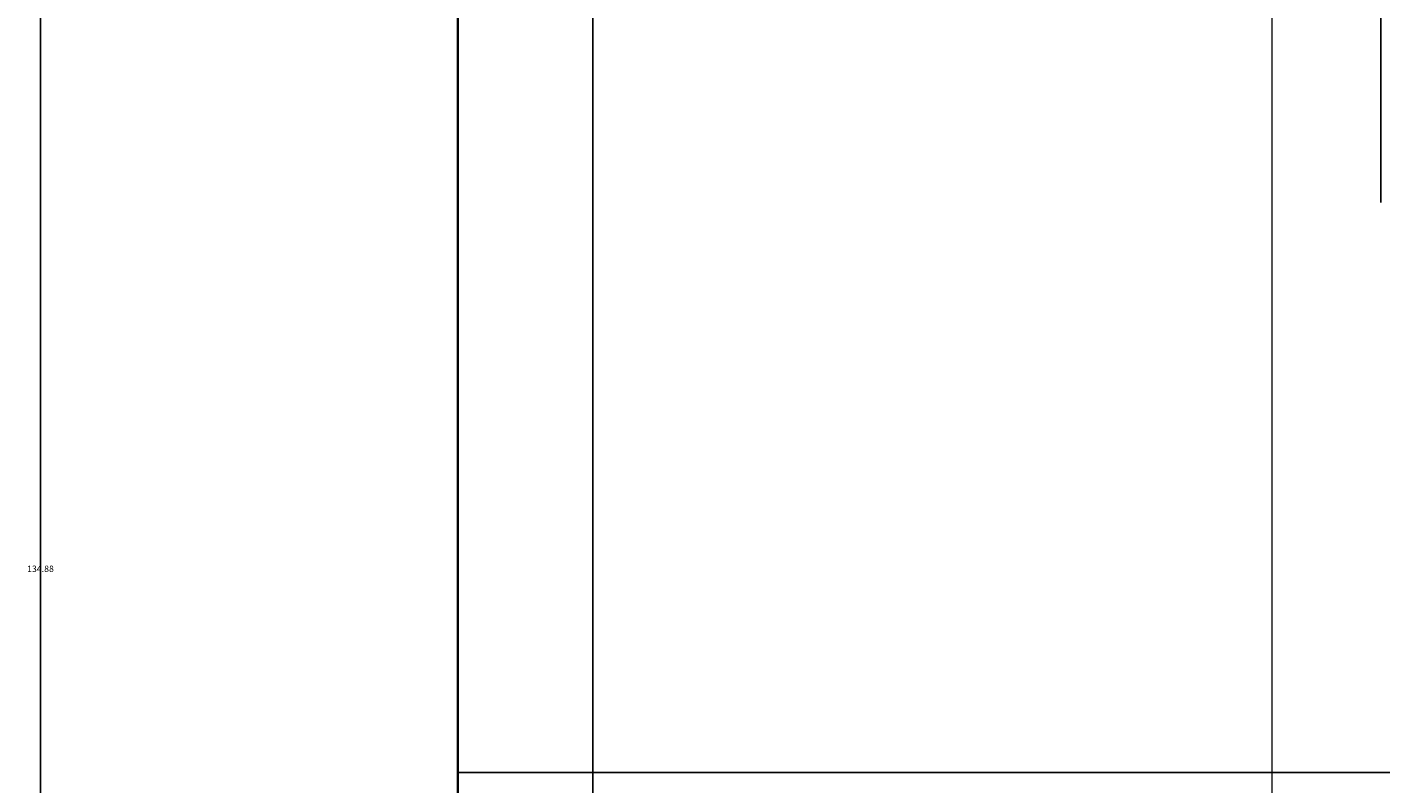
# Model space of a CAD drawing. Units: inches. Extents: x -26 to 776, y -22 to 650.
# Tile 8 of 62: x -26 to 92, y 221 to 287. Entities that reach past the tile are written whole.
import ezdxf

# ---------------------------------------------------------------- set-up
doc = ezdxf.new("R2010")
doc.units = ezdxf.units.IN
doc.header["$MEASUREMENT"] = 0
for name, color, linetype, lineweight in [('A-ANNO-DIMS', 2, 'Continuous', 18), ('A-WALL', 7, 'Continuous', 35), ('A-WALL-TRIM', 7, 'Continuous', 18)]:
    doc.layers.add(name, color=color, linetype=linetype, lineweight=lineweight)
doc.styles.get("Standard").update_dxf_attribs({"font": 'arial.ttf'})
doc.dimstyles.get("Standard").update_dxf_attribs({"dimtxt": 0.5625, "dimasz": 0.18, "dimexe": 0.18, "dimexo": 0.0625, "dimgap": 0.09, "dimtad": 0, "dimtih": 1, "dimtoh": 1, "dimdec": 4, "dimzin": 0, "dimdsep": 46, "dimlunit": 4, "dimtxsty": 'Standard', "dimcen": 0.09, "dimadec": 0, "dimazin": 0, "dimtfac": 1, "dimtdec": 4, "dimtofl": 0, "dimtmove": 0, "dimatfit": 3, "dimfxl": 1, "dimtolj": 1, "dimtzin": 0, "dimarcsym": 0})

# ---------------------------------------------------------------- blocks, each defined once
blk = doc.blocks.new('*D14')
at = {"layer": 'A-ANNO-DIMS', "color": 0, "lineweight": -2, "transparency": 16777216}
for p, q in [((191.62, 613.27), (-25.48, 613.27)), ((-25.3, 613.09), (-25.3, 314.75)), ((-25.3, 15.66), (-25.3, 314)), ((11.04, 15.48), (-25.48, 15.48))]:
    blk.add_line(p, q, dxfattribs=at)
at = {"layer": 'A-ANNO-DIMS', "color": 0, "transparency": 16777216}
for points in [[(-25.33, 613.09), (-25.27, 613.09), (-25.3, 613.27)], [(-25.33, 15.66), (-25.27, 15.66), (-25.3, 15.48)]]:
    blk.add_solid(points, dxfattribs=at)
at = {"layer": 'Defpoints', "color": 0, "transparency": 16777216}
for p in [(-25.3, 613.27), (191.68, 613.27), (11.11, 15.48)]:
    blk.add_point(p, dxfattribs=at)
at = {"layer": 'A-ANNO-DIMS', "color": 0, "transparency": 16777216, "insert": (-25.3, 314.38), "char_height": 0.562, "attachment_point": 5}
blk.add_mtext('\\A1;597.8', dxfattribs=at)
blk = doc.blocks.new('*D22')
at = {"layer": 'A-ANNO-DIMS', "color": 0, "lineweight": -2, "transparency": 16777216}
for p, q in [((22.89, 15.33), (22.89, 649.86)), ((23.07, 649.68), (119.19, 649.68)), ((217.77, 649.68), (121.65, 649.68)), ((217.95, 15.54), (217.95, 649.86))]:
    blk.add_line(p, q, dxfattribs=at)
at = {"layer": 'A-ANNO-DIMS', "color": 0, "transparency": 16777216}
for points in [[(23.07, 649.71), (23.07, 649.65), (22.89, 649.68)], [(217.77, 649.71), (217.77, 649.65), (217.95, 649.68)]]:
    blk.add_solid(points, dxfattribs=at)
at = {"layer": 'Defpoints', "color": 0, "transparency": 16777216}
for p in [(217.95, 649.68), (217.95, 15.48), (22.89, 15.27)]:
    blk.add_point(p, dxfattribs=at)
at = {"layer": 'A-ANNO-DIMS', "color": 0, "transparency": 16777216, "insert": (120.42, 649.68), "char_height": 0.562, "attachment_point": 5}
blk.add_mtext('\\A1;195.06', dxfattribs=at)
blk = doc.blocks.new('*D24')
at = {"layer": 'A-ANNO-DIMS', "color": 0, "lineweight": -2, "transparency": 16777216}
for p, q in [((11.11, 15.54), (11.11, 649.86)), ((11.29, 649.68), (15.77, 649.68)), ((22.71, 649.68), (18.23, 649.68)), ((22.89, 15.33), (22.89, 649.86))]:
    blk.add_line(p, q, dxfattribs=at)
at = {"layer": 'A-ANNO-DIMS', "color": 0, "transparency": 16777216}
for points in [[(11.29, 649.71), (11.29, 649.65), (11.11, 649.68)], [(22.71, 649.71), (22.71, 649.65), (22.89, 649.68)]]:
    blk.add_solid(points, dxfattribs=at)
at = {"layer": 'Defpoints', "color": 0, "transparency": 16777216}
for p in [(22.89, 649.68), (11.11, 15.48), (22.89, 15.27)]:
    blk.add_point(p, dxfattribs=at)
at = {"layer": 'A-ANNO-DIMS', "color": 0, "transparency": 16777216, "insert": (17, 649.68), "char_height": 0.562, "attachment_point": 5}
blk.add_mtext('\\A1;11.782', dxfattribs=at)
blk = doc.blocks.new('*D25')
at = {"layer": 'A-ANNO-DIMS', "color": 0, "lineweight": -2, "transparency": 16777216}
for p, q in [((11.11, 221.7), (11.11, 649.86)), ((11.29, 649.68), (50.34, 649.68)), ((91.46, 649.68), (52.41, 649.68)), ((91.64, 271.37), (91.64, 649.86))]:
    blk.add_line(p, q, dxfattribs=at)
at = {"layer": 'A-ANNO-DIMS', "color": 0, "transparency": 16777216}
for points in [[(11.29, 649.71), (11.29, 649.65), (11.11, 649.68)], [(91.46, 649.71), (91.46, 649.65), (91.64, 649.68)]]:
    blk.add_solid(points, dxfattribs=at)
at = {"layer": 'Defpoints', "color": 0, "transparency": 16777216}
for p in [(91.64, 649.68), (91.64, 271.31), (11.11, 221.64)]:
    blk.add_point(p, dxfattribs=at)
at = {"layer": 'A-ANNO-DIMS', "color": 0, "transparency": 16777216, "insert": (51.38, 649.68), "char_height": 0.562, "attachment_point": 5}
blk.add_mtext('\\A1;80.54', dxfattribs=at)
blk = doc.blocks.new('*D27')
at = {"layer": 'A-ANNO-DIMS', "color": 0, "lineweight": -2, "transparency": 16777216}
for p, q in [((91.58, 306.86), (-25.48, 306.86)), ((-25.3, 306.68), (-25.3, 239.79)), ((-25.3, 172.15), (-25.3, 239.04)), ((91.58, 171.97), (-25.48, 171.97))]:
    blk.add_line(p, q, dxfattribs=at)
at = {"layer": 'A-ANNO-DIMS', "color": 0, "transparency": 16777216}
for points in [[(-25.33, 306.68), (-25.27, 306.68), (-25.3, 306.86)], [(-25.33, 172.15), (-25.27, 172.15), (-25.3, 171.97)]]:
    blk.add_solid(points, dxfattribs=at)
at = {"layer": 'Defpoints', "color": 0, "transparency": 16777216}
for p in [(-25.3, 306.86), (91.64, 306.86), (91.64, 171.97)]:
    blk.add_point(p, dxfattribs=at)
at = {"layer": 'A-ANNO-DIMS', "color": 0, "transparency": 16777216, "insert": (-25.3, 239.41), "char_height": 0.562, "attachment_point": 5}
blk.add_mtext('\\A1;134.88', dxfattribs=at)
blk = doc.blocks.new('*D36')
at = {"layer": 'A-ANNO-DIMS', "color": 0, "lineweight": -2, "transparency": 16777216}
for p, q in [((82.07, 420.28), (-25.48, 420.28)), ((-25.3, 420.1), (-25.3, 290.26)), ((-25.3, 159.66), (-25.3, 289.5)), ((82.07, 159.48), (-25.48, 159.48))]:
    blk.add_line(p, q, dxfattribs=at)
at = {"layer": 'A-ANNO-DIMS', "color": 0, "transparency": 16777216}
for points in [[(-25.33, 420.1), (-25.27, 420.1), (-25.3, 420.28)], [(-25.33, 159.66), (-25.27, 159.66), (-25.3, 159.48)]]:
    blk.add_solid(points, dxfattribs=at)
at = {"layer": 'Defpoints', "color": 0, "transparency": 16777216}
for p in [(-25.3, 420.28), (82.13, 420.28), (82.13, 159.48)]:
    blk.add_point(p, dxfattribs=at)
at = {"layer": 'A-ANNO-DIMS', "color": 0, "transparency": 16777216, "insert": (-25.3, 289.88), "char_height": 0.562, "attachment_point": 5}
blk.add_mtext('\\A1;260.8', dxfattribs=at)
blk = doc.blocks.new('*D41')
at = {"layer": 'A-ANNO-DIMS', "color": 0, "lineweight": -2, "transparency": 16777216}
for p, q in [((11.17, 221.64), (775.34, 221.64)), ((775.16, 221.46), (775.16, 190.94)), ((775.16, 159.66), (775.16, 190.18)), ((11.17, 159.48), (775.34, 159.48))]:
    blk.add_line(p, q, dxfattribs=at)
at = {"layer": 'A-ANNO-DIMS', "color": 0, "transparency": 16777216}
for points in [[(775.13, 221.46), (775.19, 221.46), (775.16, 221.64)], [(775.13, 159.66), (775.19, 159.66), (775.16, 159.48)]]:
    blk.add_solid(points, dxfattribs=at)
at = {"layer": 'Defpoints', "color": 0, "transparency": 16777216}
for p in [(11.11, 221.64), (775.16, 221.64), (11.11, 159.48)]:
    blk.add_point(p, dxfattribs=at)
at = {"layer": 'A-ANNO-DIMS', "color": 0, "transparency": 16777216, "insert": (775.16, 190.56), "char_height": 0.562, "attachment_point": 5}
blk.add_mtext('\\A1;62.16', dxfattribs=at)

msp = doc.modelspace()

# ---------------------------------------------------------------- linework, layer by layer
at = {"layer": 'A-WALL'}
msp.add_line((11.1074, 159.4824), (11.1074, 338.1203), dxfattribs=at)
at = {"layer": 'A-WALL-TRIM'}
msp.add_line((11.1074, 221.6413), (82.134, 221.6413), dxfattribs=at)
msp.add_lwpolyline([(82.134, 159.4824), (209.091, 159.4824), (209.091, 420.2783), (82.134, 420.2783)], close=True, dxfattribs=at)

# ---------------------------------------------------------------- dimensions: what is measured, and where the dimension line sits
at = {"layer": 'A-ANNO-DIMS'}
for base, p1, p2, override, picture, middle in [((22.8891, 649.6763), (11.1074, 15.4824), (22.8891, 15.2701), {"dimdec": 3, "dimlfac": 1, "dimrnd": 0, "dimzin": 0, "dimdsep": 46, "dimlunit": 2}, '*D24', (16.9982, 649.6763)), ((91.6448, 649.6763), (11.1074, 221.6413), (91.6448, 271.3091), {"dimdec": 2, "dimlfac": 1, "dimrnd": 0, "dimzin": 0, "dimdsep": 46, "dimlunit": 2}, '*D25', (51.3761, 649.6763)), ((217.9529, 649.6763), (22.8891, 15.2701), (217.9529, 15.4824), {"dimdec": 2, "dimlfac": 1, "dimrnd": 0, "dimzin": 0, "dimdsep": 46, "dimlunit": 2}, '*D22', (120.421, 649.6763))]:
    dim = msp.add_linear_dim(base=base, p1=p1, p2=p2, dimstyle='Standard', override=override, dxfattribs=at)
    dim.commit()
    dim.dimension.update_dxf_attribs({"geometry": picture, "text_midpoint": middle})
for base, p1, p2, override, picture, middle in [((-25.2976, 613.2713), (11.1074, 15.4824), (191.6782, 613.2713), {"dimdec": 1, "dimlfac": 1, "dimrnd": 0, "dimzin": 0, "dimdsep": 46, "dimlunit": 2}, '*D14', (-25.2976, 314.3769)), ((-25.2976, 420.2783), (82.134, 159.4824), (82.134, 420.2783), {"dimdec": 1, "dimlfac": 1, "dimrnd": 0, "dimzin": 0, "dimdsep": 46, "dimlunit": 2}, '*D36', (-25.2976, 289.8803)), ((-25.2976, 306.8552), (91.6448, 171.9734), (91.6448, 306.8552), {"dimdec": 2, "dimlfac": 1, "dimrnd": 0, "dimzin": 0, "dimdsep": 46, "dimlunit": 2}, '*D27', (-25.2976, 239.4143)), ((775.1553, 221.6413), (11.1074, 159.4824), (11.1074, 221.6413), {"dimdec": 2, "dimlfac": 1, "dimrnd": 0, "dimzin": 0, "dimdsep": 46, "dimlunit": 2}, '*D41', (775.1553, 190.5618))]:
    dim = msp.add_linear_dim(base=base, p1=p1, p2=p2, angle=90, dimstyle='Standard', override=override, dxfattribs=at)
    dim.commit()
    dim.dimension.update_dxf_attribs({"geometry": picture, "text_midpoint": middle})

doc.saveas('drawing.dxf')
